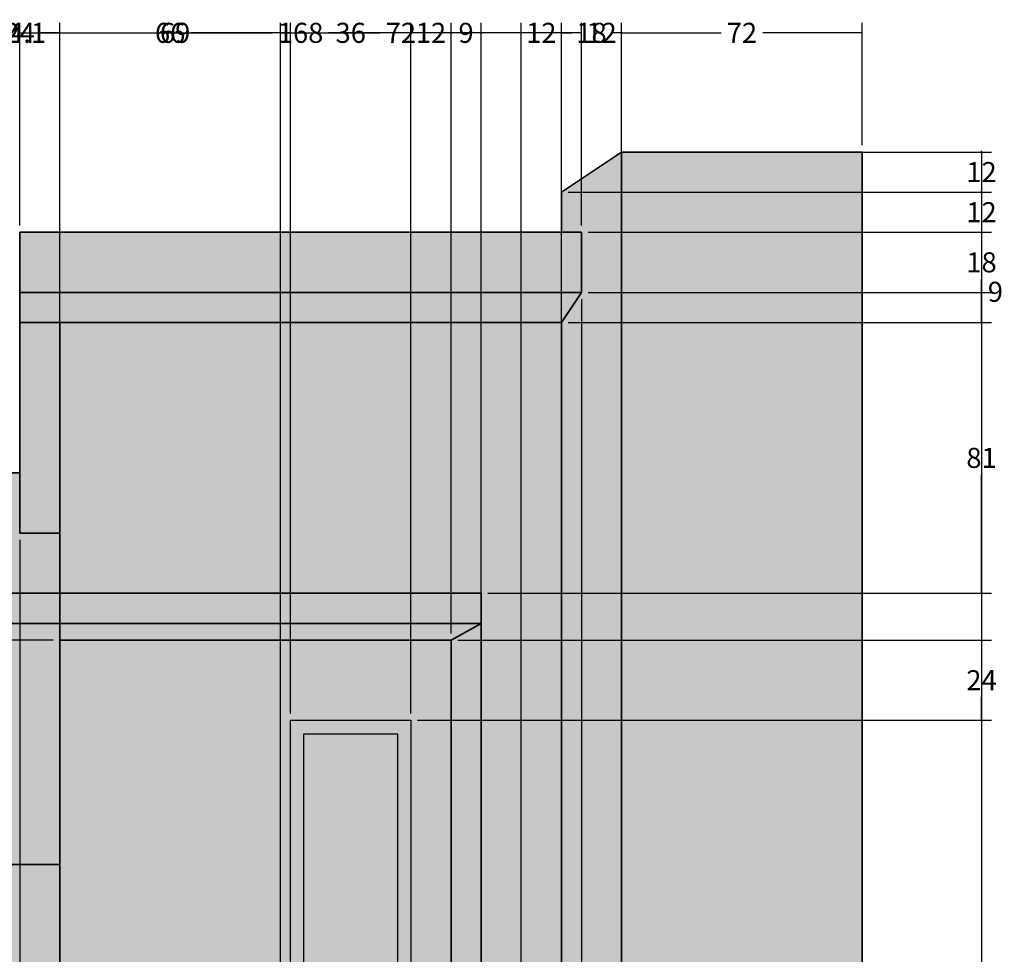
# Model space of a CAD drawing. Units: inches. Extents: x 860 to 1491, y 583 to 1370.
# Tile 8 of 8: x 1190 to 1485, y 1091 to 1370. Entities that reach past the tile are written whole.
import ezdxf

# ---------------------------------------------------------------- set-up
doc = ezdxf.new("R2010")
doc.units = ezdxf.units.IN
doc.header["$MEASUREMENT"] = 0
doc.layers.get('0').update_dxf_attribs({"color": 250})
for name, color, linetype, lineweight in [('A-ANNO-DIMS', 2, 'Continuous', 18), ('A-ELEV', 7, 'Continuous', 35), ('A-ELEV-PATT', 9, 'Continuous', 13), ('A-GLAZ', 4, 'Continuous', 25), ('A-GLAZ-PATT', 150, 'Continuous', 13)]:
    doc.layers.add(name, color=color, linetype=linetype, lineweight=lineweight)
doc.styles.get("Standard").update_dxf_attribs({"font": 'arial.ttf'})
doc.dimstyles.get("Standard").update_dxf_attribs({"dimtxt": 6, "dimasz": 0.18, "dimexe": 3, "dimexo": 2, "dimgap": 2, "dimtad": 0, "dimtih": 1, "dimtoh": 1, "dimdec": 0, "dimzin": 0, "dimdsep": 46, "dimlunit": 3, "dimtxsty": 'Standard', "dimblk2": 'CLOSEDBLANK', "dimsah": 1, "dimcen": 2, "dimadec": 0, "dimazin": 0, "dimtfac": 1, "dimtdec": 0, "dimtofl": 0, "dimtmove": 0, "dimatfit": 3, "dimfxl": 1, "dimtolj": 1, "dimtzin": 0, "dimarcsym": 0})

# ---------------------------------------------------------------- blocks, each defined once
blk = doc.blocks.new('_ClosedBlank')
at = {"color": 0, "linetype": 'ByBlock', "lineweight": -2}
for p, q in [((-1, 0.17), (0, 0)), ((-1, 0.17), (-1, -0.17)), ((0, 0), (-1, -0.17))]:
    blk.add_line(p, q, dxfattribs=at)
blk = doc.blocks.new('*D2')
at = {"layer": 'A-ANNO-DIMS', "color": 0, "lineweight": -2, "transparency": 16777216}
for p, q in [((1442.44, 1328.76), (1442.44, 584.11)), ((908.34, 740.76), (908.34, 584.11)), ((908.52, 587.11), (1163.85, 587.11)), ((1442.26, 587.11), (1186.93, 587.11))]:
    blk.add_line(p, q, dxfattribs=at)
at = {"layer": 'A-ANNO-DIMS', "color": 0, "transparency": 16777216}
blk.add_solid([(908.52, 587.14), (908.52, 587.08), (908.34, 587.11)], dxfattribs=at)
at = {"layer": 'Defpoints', "color": 0, "transparency": 16777216}
for p in [(1442.44, 1330.76), (908.34, 742.76), (1442.44, 587.11)]:
    blk.add_point(p, dxfattribs=at)
at = {"layer": 'A-ANNO-DIMS', "color": 0, "lineweight": -2, "transparency": 16777216, "xscale": 0.18, "yscale": 0.18, "zscale": 0.18}
blk.add_blockref('_ClosedBlank', (1442.44, 587.11), dxfattribs=at)
at = {"layer": 'A-ANNO-DIMS', "color": 0, "transparency": 16777216, "insert": (1175.39, 587.11), "char_height": 6, "attachment_point": 5}
blk.add_mtext('\\A1;534.1', dxfattribs=at)
blk = doc.blocks.new('*D3')
at = {"layer": 'A-ANNO-DIMS', "color": 0, "lineweight": -2, "transparency": 16777216}
for p, q in [((1444.44, 1330.76), (1481.09, 1330.76)), ((1478.09, 1330.58), (1478.09, 981.82)), ((1478.09, 622.94), (1478.09, 971.69)), ((1444.44, 622.76), (1481.09, 622.76))]:
    blk.add_line(p, q, dxfattribs=at)
at = {"layer": 'A-ANNO-DIMS', "color": 0, "transparency": 16777216}
blk.add_solid([(1478.06, 622.94), (1478.12, 622.94), (1478.09, 622.76)], dxfattribs=at)
at = {"layer": 'Defpoints', "color": 0, "transparency": 16777216}
for p in [(1442.44, 1330.76), (1478.09, 1330.76), (1442.44, 622.76)]:
    blk.add_point(p, dxfattribs=at)
at = {"layer": 'A-ANNO-DIMS', "color": 0, "lineweight": -2, "transparency": 16777216, "xscale": 0.18, "yscale": 0.18, "zscale": 0.18, "rotation": 90}
blk.add_blockref('_ClosedBlank', (1478.09, 1330.76), dxfattribs=at)
at = {"layer": 'A-ANNO-DIMS', "color": 0, "transparency": 16777216, "insert": (1478.09, 976.76), "char_height": 6, "attachment_point": 5}
blk.add_mtext('\\A1;708', dxfattribs=at)
blk = doc.blocks.new('*D25')
at = {"layer": 'A-ANNO-DIMS', "color": 0, "lineweight": -2, "transparency": 16777216}
for p, q in [((1178.44, 840.76), (1178.44, 1369.41)), ((1202.44, 744.76), (1202.44, 1369.41)), ((1178.62, 1366.41), (1184.1, 1366.41)), ((1202.26, 1366.41), (1196.78, 1366.41))]:
    blk.add_line(p, q, dxfattribs=at)
at = {"layer": 'A-ANNO-DIMS', "color": 0, "transparency": 16777216}
blk.add_solid([(1178.62, 1366.44), (1178.62, 1366.38), (1178.44, 1366.41)], dxfattribs=at)
at = {"layer": 'Defpoints', "color": 0, "transparency": 16777216}
for p in [(1202.44, 1366.41), (1178.44, 838.76), (1202.44, 742.76)]:
    blk.add_point(p, dxfattribs=at)
at = {"layer": 'A-ANNO-DIMS', "color": 0, "lineweight": -2, "transparency": 16777216, "xscale": 0.18, "yscale": 0.18, "zscale": 0.18}
blk.add_blockref('_ClosedBlank', (1202.44, 1366.41), dxfattribs=at)
at = {"layer": 'A-ANNO-DIMS', "color": 0, "transparency": 16777216, "insert": (1190.44, 1366.41), "char_height": 6, "attachment_point": 5}
blk.add_mtext('\\A1;24', dxfattribs=at)
blk = doc.blocks.new('*D26')
at = {"layer": 'A-ANNO-DIMS', "color": 0, "lineweight": -2, "transparency": 16777216}
for p, q in [((1202.44, 744.76), (1202.44, 1369.41)), ((1268.44, 864.76), (1268.44, 1369.41)), ((1202.62, 1366.41), (1229.13, 1366.41)), ((1268.26, 1366.41), (1241.75, 1366.41))]:
    blk.add_line(p, q, dxfattribs=at)
at = {"layer": 'A-ANNO-DIMS', "color": 0, "transparency": 16777216}
blk.add_solid([(1202.62, 1366.44), (1202.62, 1366.38), (1202.44, 1366.41)], dxfattribs=at)
at = {"layer": 'Defpoints', "color": 0, "transparency": 16777216}
for p in [(1268.44, 1366.41), (1268.44, 862.76), (1202.44, 742.76)]:
    blk.add_point(p, dxfattribs=at)
at = {"layer": 'A-ANNO-DIMS', "color": 0, "lineweight": -2, "transparency": 16777216, "xscale": 0.18, "yscale": 0.18, "zscale": 0.18}
blk.add_blockref('_ClosedBlank', (1268.44, 1366.41), dxfattribs=at)
at = {"layer": 'A-ANNO-DIMS', "color": 0, "transparency": 16777216, "insert": (1235.44, 1366.41), "char_height": 6, "attachment_point": 5}
blk.add_mtext('\\A1;66', dxfattribs=at)
blk = doc.blocks.new('*D27')
at = {"layer": 'A-ANNO-DIMS', "color": 0, "lineweight": -2, "transparency": 16777216}
for p, q in [((1268.44, 864.76), (1268.44, 1369.41)), ((1340.44, 864.76), (1340.44, 1369.41)), ((1268.62, 1366.41), (1298.2, 1366.41)), ((1340.26, 1366.41), (1310.68, 1366.41))]:
    blk.add_line(p, q, dxfattribs=at)
at = {"layer": 'A-ANNO-DIMS', "color": 0, "transparency": 16777216}
blk.add_solid([(1268.62, 1366.44), (1268.62, 1366.38), (1268.44, 1366.41)], dxfattribs=at)
at = {"layer": 'Defpoints', "color": 0, "transparency": 16777216}
for p in [(1340.44, 1366.41), (1268.44, 862.76), (1340.44, 862.76)]:
    blk.add_point(p, dxfattribs=at)
at = {"layer": 'A-ANNO-DIMS', "color": 0, "lineweight": -2, "transparency": 16777216, "xscale": 0.18, "yscale": 0.18, "zscale": 0.18}
blk.add_blockref('_ClosedBlank', (1340.44, 1366.41), dxfattribs=at)
at = {"layer": 'A-ANNO-DIMS', "color": 0, "transparency": 16777216, "insert": (1304.44, 1366.41), "char_height": 6, "attachment_point": 5}
blk.add_mtext('\\A1;72', dxfattribs=at)
blk = doc.blocks.new('*D28')
at = {"layer": 'A-ANNO-DIMS', "color": 0, "lineweight": -2, "transparency": 16777216}
for p, q in [((1340.440309, 864.755507), (1340.440309, 1369.405507)), ((1352.440309, 732.755507), (1352.440309, 1369.405507)), ((1340.260309, 1366.405507), (1340.080309, 1366.405507)), ((1352.620309, 1366.405507), (1352.800309, 1366.405507))]:
    blk.add_line(p, q, dxfattribs=at)
at = {"layer": 'A-ANNO-DIMS', "color": 0, "transparency": 16777216}
blk.add_solid([(1340.260309, 1366.435507), (1340.260309, 1366.375507), (1340.440309, 1366.405507)], dxfattribs=at)
at = {"layer": 'Defpoints', "color": 0, "transparency": 16777216}
for p in [(1352.440309, 1366.405507), (1340.440309, 862.755507), (1352.440309, 730.755507)]:
    blk.add_point(p, dxfattribs=at)
at = {"layer": 'A-ANNO-DIMS', "color": 0, "lineweight": -2, "transparency": 16777216, "xscale": 0.18, "yscale": 0.18, "zscale": 0.18, "rotation": 180}
blk.add_blockref('_ClosedBlank', (1352.440309, 1366.405507), dxfattribs=at)
at = {"layer": 'A-ANNO-DIMS', "color": 0, "transparency": 16777216, "insert": (1346.440309, 1366.405507), "char_height": 6, "attachment_point": 5}
blk.add_mtext('\\A1;12', dxfattribs=at)
blk = doc.blocks.new('*D29')
at = {"layer": 'A-ANNO-DIMS', "color": 0, "lineweight": -2, "transparency": 16777216}
for p, q in [((1352.44, 732.76), (1352.44, 1369.41)), ((1370.44, 732.76), (1370.44, 1369.41)), ((1352.62, 1366.41), (1355.42, 1366.41)), ((1370.26, 1366.41), (1367.46, 1366.41))]:
    blk.add_line(p, q, dxfattribs=at)
at = {"layer": 'A-ANNO-DIMS', "color": 0, "transparency": 16777216}
blk.add_solid([(1352.62, 1366.44), (1352.62, 1366.38), (1352.44, 1366.41)], dxfattribs=at)
at = {"layer": 'Defpoints', "color": 0, "transparency": 16777216}
for p in [(1370.44, 1366.41), (1352.44, 730.76), (1370.44, 730.76)]:
    blk.add_point(p, dxfattribs=at)
at = {"layer": 'A-ANNO-DIMS', "color": 0, "lineweight": -2, "transparency": 16777216, "xscale": 0.18, "yscale": 0.18, "zscale": 0.18}
blk.add_blockref('_ClosedBlank', (1370.44, 1366.41), dxfattribs=at)
at = {"layer": 'A-ANNO-DIMS', "color": 0, "transparency": 16777216, "insert": (1361.44, 1366.41), "char_height": 6, "attachment_point": 5}
blk.add_mtext('\\A1;18', dxfattribs=at)
blk = doc.blocks.new('*D47')
at = {"layer": 'A-ANNO-DIMS', "color": 0, "lineweight": -2, "transparency": 16777216}
for p, q in [((1200.44, 1184.76), (869.69, 1184.76)), ((872.69, 1184.58), (872.69, 1156.25)), ((872.69, 1117.8), (872.69, 1146.12)), ((960.34, 1117.62), (869.69, 1117.62))]:
    blk.add_line(p, q, dxfattribs=at)
at = {"layer": 'A-ANNO-DIMS', "color": 0, "transparency": 16777216}
blk.add_solid([(872.66, 1117.8), (872.72, 1117.8), (872.69, 1117.62)], dxfattribs=at)
at = {"layer": 'Defpoints', "color": 0, "transparency": 16777216}
for p in [(872.69, 1184.76), (1202.44, 1184.76), (962.34, 1117.62)]:
    blk.add_point(p, dxfattribs=at)
at = {"layer": 'A-ANNO-DIMS', "color": 0, "lineweight": -2, "transparency": 16777216, "xscale": 0.18, "yscale": 0.18, "zscale": 0.18, "rotation": 90}
blk.add_blockref('_ClosedBlank', (872.69, 1184.76), dxfattribs=at)
at = {"layer": 'A-ANNO-DIMS', "color": 0, "transparency": 16777216, "insert": (872.69, 1151.19), "char_height": 6, "attachment_point": 5}
blk.add_mtext('\\A1;67.13', dxfattribs=at)
blk = doc.blocks.new('*D53')
at = {"layer": 'A-ANNO-DIMS', "color": 0, "lineweight": -2, "transparency": 16777216}
for p, q in [((1309.44, 1160.76), (1481.09, 1160.76)), ((1478.09, 1160.58), (1478.09, 1057.82)), ((1478.09, 944.94), (1478.09, 1047.69)), ((1309.44, 944.76), (1481.09, 944.76))]:
    blk.add_line(p, q, dxfattribs=at)
at = {"layer": 'A-ANNO-DIMS', "color": 0, "transparency": 16777216}
blk.add_solid([(1478.06, 944.94), (1478.12, 944.94), (1478.09, 944.76)], dxfattribs=at)
at = {"layer": 'Defpoints', "color": 0, "transparency": 16777216}
for p in [(1307.44, 1160.76), (1478.09, 1160.76), (1307.44, 944.76)]:
    blk.add_point(p, dxfattribs=at)
at = {"layer": 'A-ANNO-DIMS', "color": 0, "lineweight": -2, "transparency": 16777216, "xscale": 0.18, "yscale": 0.18, "zscale": 0.18, "rotation": 90}
blk.add_blockref('_ClosedBlank', (1478.09, 1160.76), dxfattribs=at)
at = {"layer": 'A-ANNO-DIMS', "color": 0, "transparency": 16777216, "insert": (1478.09, 1052.76), "char_height": 6, "attachment_point": 5}
blk.add_mtext('\\A1;216', dxfattribs=at)
blk = doc.blocks.new('*D54')
at = {"layer": 'A-ANNO-DIMS', "color": 0, "lineweight": -2, "transparency": 16777216}
for p, q in [((1321.44, 1184.76), (1481.09, 1184.76)), ((1478.09, 1184.58), (1478.09, 1177.77)), ((1478.09, 1160.94), (1478.09, 1167.74)), ((1309.44, 1160.76), (1481.09, 1160.76))]:
    blk.add_line(p, q, dxfattribs=at)
at = {"layer": 'A-ANNO-DIMS', "color": 0, "transparency": 16777216}
blk.add_solid([(1478.06, 1160.94), (1478.12, 1160.94), (1478.09, 1160.76)], dxfattribs=at)
at = {"layer": 'Defpoints', "color": 0, "transparency": 16777216}
for p in [(1319.44, 1184.76), (1478.09, 1184.76), (1307.44, 1160.76)]:
    blk.add_point(p, dxfattribs=at)
at = {"layer": 'A-ANNO-DIMS', "color": 0, "lineweight": -2, "transparency": 16777216, "xscale": 0.18, "yscale": 0.18, "zscale": 0.18, "rotation": 90}
blk.add_blockref('_ClosedBlank', (1478.09, 1184.76), dxfattribs=at)
at = {"layer": 'A-ANNO-DIMS', "color": 0, "transparency": 16777216, "insert": (1478.09, 1172.76), "char_height": 6, "attachment_point": 5}
blk.add_mtext('\\A1;24', dxfattribs=at)
blk = doc.blocks.new('*D57')
at = {"layer": 'A-ANNO-DIMS', "color": 0, "lineweight": -2, "transparency": 16777216}
for p, q in [((1178.34, 1092.76), (1178.34, 1369.41)), ((1202.44, 1186.76), (1202.44, 1369.41)), ((1178.52, 1366.41), (1181.13, 1366.41)), ((1202.26, 1366.41), (1199.65, 1366.41))]:
    blk.add_line(p, q, dxfattribs=at)
at = {"layer": 'A-ANNO-DIMS', "color": 0, "transparency": 16777216}
blk.add_solid([(1178.52, 1366.44), (1178.52, 1366.38), (1178.34, 1366.41)], dxfattribs=at)
at = {"layer": 'Defpoints', "color": 0, "transparency": 16777216}
for p in [(1202.44, 1366.41), (1202.44, 1184.76), (1178.34, 1090.76)]:
    blk.add_point(p, dxfattribs=at)
at = {"layer": 'A-ANNO-DIMS', "color": 0, "lineweight": -2, "transparency": 16777216, "xscale": 0.18, "yscale": 0.18, "zscale": 0.18}
blk.add_blockref('_ClosedBlank', (1202.44, 1366.41), dxfattribs=at)
at = {"layer": 'A-ANNO-DIMS', "color": 0, "transparency": 16777216, "insert": (1190.39, 1366.41), "char_height": 6, "attachment_point": 5}
blk.add_mtext('\\A1;24.1', dxfattribs=at)
blk = doc.blocks.new('*D58')
at = {"layer": 'A-ANNO-DIMS', "color": 0, "lineweight": -2, "transparency": 16777216}
for p, q in [((1202.44, 1186.76), (1202.44, 1369.41)), ((1271.44, 1162.76), (1271.44, 1369.41)), ((1202.62, 1366.41), (1230.62, 1366.41)), ((1271.26, 1366.41), (1243.26, 1366.41))]:
    blk.add_line(p, q, dxfattribs=at)
at = {"layer": 'A-ANNO-DIMS', "color": 0, "transparency": 16777216}
blk.add_solid([(1202.62, 1366.44), (1202.62, 1366.38), (1202.44, 1366.41)], dxfattribs=at)
at = {"layer": 'Defpoints', "color": 0, "transparency": 16777216}
for p in [(1271.44, 1366.41), (1202.44, 1184.76), (1271.44, 1160.76)]:
    blk.add_point(p, dxfattribs=at)
at = {"layer": 'A-ANNO-DIMS', "color": 0, "lineweight": -2, "transparency": 16777216, "xscale": 0.18, "yscale": 0.18, "zscale": 0.18}
blk.add_blockref('_ClosedBlank', (1271.44, 1366.41), dxfattribs=at)
at = {"layer": 'A-ANNO-DIMS', "color": 0, "transparency": 16777216, "insert": (1236.94, 1366.41), "char_height": 6, "attachment_point": 5}
blk.add_mtext('\\A1;69', dxfattribs=at)
blk = doc.blocks.new('*D59')
at = {"layer": 'A-ANNO-DIMS', "color": 0, "lineweight": -2, "transparency": 16777216}
for p, q in [((1271.44, 1162.76), (1271.44, 1369.41)), ((1307.44, 1162.76), (1307.44, 1369.41)), ((1271.62, 1366.41), (1283.15, 1366.41)), ((1307.26, 1366.41), (1295.73, 1366.41))]:
    blk.add_line(p, q, dxfattribs=at)
at = {"layer": 'A-ANNO-DIMS', "color": 0, "transparency": 16777216}
blk.add_solid([(1271.62, 1366.44), (1271.62, 1366.38), (1271.44, 1366.41)], dxfattribs=at)
at = {"layer": 'Defpoints', "color": 0, "transparency": 16777216}
for p in [(1307.44, 1366.41), (1271.44, 1160.76), (1307.44, 1160.76)]:
    blk.add_point(p, dxfattribs=at)
at = {"layer": 'A-ANNO-DIMS', "color": 0, "lineweight": -2, "transparency": 16777216, "xscale": 0.18, "yscale": 0.18, "zscale": 0.18}
blk.add_blockref('_ClosedBlank', (1307.44, 1366.41), dxfattribs=at)
at = {"layer": 'A-ANNO-DIMS', "color": 0, "transparency": 16777216, "insert": (1289.44, 1366.41), "char_height": 6, "attachment_point": 5}
blk.add_mtext('\\A1;36', dxfattribs=at)
blk = doc.blocks.new('*D60')
at = {"layer": 'A-ANNO-DIMS', "color": 0, "lineweight": -2, "transparency": 16777216}
for p, q in [((1307.440309, 1162.755507), (1307.440309, 1369.405507)), ((1319.440309, 1186.755507), (1319.440309, 1369.405507)), ((1307.260309, 1366.405507), (1307.080309, 1366.405507)), ((1319.620309, 1366.405507), (1319.800309, 1366.405507))]:
    blk.add_line(p, q, dxfattribs=at)
at = {"layer": 'A-ANNO-DIMS', "color": 0, "transparency": 16777216}
blk.add_solid([(1307.260309, 1366.435507), (1307.260309, 1366.375507), (1307.440309, 1366.405507)], dxfattribs=at)
at = {"layer": 'Defpoints', "color": 0, "transparency": 16777216}
for p in [(1319.440309, 1366.405507), (1319.440309, 1184.755507), (1307.440309, 1160.755507)]:
    blk.add_point(p, dxfattribs=at)
at = {"layer": 'A-ANNO-DIMS', "color": 0, "lineweight": -2, "transparency": 16777216, "xscale": 0.18, "yscale": 0.18, "zscale": 0.18, "rotation": 180}
blk.add_blockref('_ClosedBlank', (1319.440309, 1366.405507), dxfattribs=at)
at = {"layer": 'A-ANNO-DIMS', "color": 0, "transparency": 16777216, "insert": (1313.440309, 1366.405507), "char_height": 6, "attachment_point": 5}
blk.add_mtext('\\A1;12', dxfattribs=at)
blk = doc.blocks.new('*D61')
at = {"layer": 'A-ANNO-DIMS', "color": 0, "lineweight": -2, "transparency": 16777216}
for p, q in [((1319.440309, 1186.755507), (1319.440309, 1369.405507)), ((1328.440309, 924.755507), (1328.440309, 1369.405507)), ((1319.260309, 1366.405507), (1319.080309, 1366.405507)), ((1328.620309, 1366.405507), (1328.800309, 1366.405507))]:
    blk.add_line(p, q, dxfattribs=at)
at = {"layer": 'A-ANNO-DIMS', "color": 0, "transparency": 16777216}
blk.add_solid([(1319.260309, 1366.435507), (1319.260309, 1366.375507), (1319.440309, 1366.405507)], dxfattribs=at)
at = {"layer": 'Defpoints', "color": 0, "transparency": 16777216}
for p in [(1328.440309, 1366.405507), (1319.440309, 1184.755507), (1328.440309, 922.755507)]:
    blk.add_point(p, dxfattribs=at)
at = {"layer": 'A-ANNO-DIMS', "color": 0, "lineweight": -2, "transparency": 16777216, "xscale": 0.18, "yscale": 0.18, "zscale": 0.18, "rotation": 180}
blk.add_blockref('_ClosedBlank', (1328.440309, 1366.405507), dxfattribs=at)
at = {"layer": 'A-ANNO-DIMS', "color": 0, "transparency": 16777216, "insert": (1323.940309, 1366.405507), "char_height": 6, "attachment_point": 5}
blk.add_mtext('\\A1;9', dxfattribs=at)
blk = doc.blocks.new('*D73')
at = {"layer": 'A-ANNO-DIMS', "color": 0, "lineweight": -2, "transparency": 16777216}
for p, q in [((1190.44, 1308.76), (1190.44, 1369.41)), ((1358.44, 1308.76), (1358.44, 1369.41)), ((1190.62, 1366.41), (1266.09, 1366.41)), ((1358.26, 1366.41), (1282.79, 1366.41))]:
    blk.add_line(p, q, dxfattribs=at)
at = {"layer": 'A-ANNO-DIMS', "color": 0, "transparency": 16777216}
blk.add_solid([(1190.62, 1366.44), (1190.62, 1366.38), (1190.44, 1366.41)], dxfattribs=at)
at = {"layer": 'Defpoints', "color": 0, "transparency": 16777216}
for p in [(1358.44, 1366.41), (1190.44, 1306.76), (1358.44, 1306.76)]:
    blk.add_point(p, dxfattribs=at)
at = {"layer": 'A-ANNO-DIMS', "color": 0, "lineweight": -2, "transparency": 16777216, "xscale": 0.18, "yscale": 0.18, "zscale": 0.18}
blk.add_blockref('_ClosedBlank', (1358.44, 1366.41), dxfattribs=at)
at = {"layer": 'A-ANNO-DIMS', "color": 0, "transparency": 16777216, "insert": (1274.44, 1366.41), "char_height": 6, "attachment_point": 5}
blk.add_mtext('\\A1;168', dxfattribs=at)
blk = doc.blocks.new('*D74')
at = {"layer": 'A-ANNO-DIMS', "color": 0, "lineweight": -2, "transparency": 16777216}
for p, q in [((1358.440309, 1308.755507), (1358.440309, 1369.405507)), ((1370.440309, 1332.755507), (1370.440309, 1369.405507)), ((1358.260309, 1366.405507), (1358.080309, 1366.405507)), ((1370.620309, 1366.405507), (1370.800309, 1366.405507))]:
    blk.add_line(p, q, dxfattribs=at)
at = {"layer": 'A-ANNO-DIMS', "color": 0, "transparency": 16777216}
blk.add_solid([(1358.260309, 1366.435507), (1358.260309, 1366.375507), (1358.440309, 1366.405507)], dxfattribs=at)
at = {"layer": 'Defpoints', "color": 0, "transparency": 16777216}
for p in [(1370.440309, 1366.405507), (1370.440309, 1330.755507), (1358.440309, 1306.755507)]:
    blk.add_point(p, dxfattribs=at)
at = {"layer": 'A-ANNO-DIMS', "color": 0, "lineweight": -2, "transparency": 16777216, "xscale": 0.18, "yscale": 0.18, "zscale": 0.18, "rotation": 180}
blk.add_blockref('_ClosedBlank', (1370.440309, 1366.405507), dxfattribs=at)
at = {"layer": 'A-ANNO-DIMS', "color": 0, "transparency": 16777216, "insert": (1364.440309, 1366.405507), "char_height": 6, "attachment_point": 5}
blk.add_mtext('\\A1;12', dxfattribs=at)
blk = doc.blocks.new('*D75')
at = {"layer": 'A-ANNO-DIMS', "color": 0, "lineweight": -2, "transparency": 16777216}
for p, q in [((1370.44, 1332.76), (1370.44, 1369.41)), ((1442.44, 1332.76), (1442.44, 1369.41)), ((1370.62, 1366.41), (1400.2, 1366.41)), ((1442.26, 1366.41), (1412.68, 1366.41))]:
    blk.add_line(p, q, dxfattribs=at)
at = {"layer": 'A-ANNO-DIMS', "color": 0, "transparency": 16777216}
blk.add_solid([(1370.62, 1366.44), (1370.62, 1366.38), (1370.44, 1366.41)], dxfattribs=at)
at = {"layer": 'Defpoints', "color": 0, "transparency": 16777216}
for p in [(1442.44, 1366.41), (1370.44, 1330.76), (1442.44, 1330.76)]:
    blk.add_point(p, dxfattribs=at)
at = {"layer": 'A-ANNO-DIMS', "color": 0, "lineweight": -2, "transparency": 16777216, "xscale": 0.18, "yscale": 0.18, "zscale": 0.18}
blk.add_blockref('_ClosedBlank', (1442.44, 1366.41), dxfattribs=at)
at = {"layer": 'A-ANNO-DIMS', "color": 0, "transparency": 16777216, "insert": (1406.44, 1366.41), "char_height": 6, "attachment_point": 5}
blk.add_mtext('\\A1;72', dxfattribs=at)
blk = doc.blocks.new('*D76')
at = {"layer": 'A-ANNO-DIMS', "color": 0, "lineweight": -2, "transparency": 16777216}
for p, q in [((1202.440309, 1277.755507), (1202.440309, 584.105507)), ((1190.440309, 1214.755507), (1190.440309, 584.105507)), ((1190.260309, 587.105507), (1190.080309, 587.105507)), ((1202.620309, 587.105507), (1202.800309, 587.105507))]:
    blk.add_line(p, q, dxfattribs=at)
at = {"layer": 'A-ANNO-DIMS', "color": 0, "transparency": 16777216}
blk.add_solid([(1190.260309, 587.135507), (1190.260309, 587.075507), (1190.440309, 587.105507)], dxfattribs=at)
at = {"layer": 'Defpoints', "color": 0, "transparency": 16777216}
for p in [(1202.440309, 1279.755507), (1190.440309, 1216.755507), (1202.440309, 587.105507)]:
    blk.add_point(p, dxfattribs=at)
at = {"layer": 'A-ANNO-DIMS', "color": 0, "lineweight": -2, "transparency": 16777216, "xscale": 0.18, "yscale": 0.18, "zscale": 0.18, "rotation": 180}
blk.add_blockref('_ClosedBlank', (1202.440309, 587.105507), dxfattribs=at)
at = {"layer": 'A-ANNO-DIMS', "color": 0, "transparency": 16777216, "insert": (1196.440309, 587.105507), "char_height": 6, "attachment_point": 5}
blk.add_mtext('\\A1;12', dxfattribs=at)
blk = doc.blocks.new('*D77')
at = {"layer": 'A-ANNO-DIMS', "color": 0, "lineweight": -2, "transparency": 16777216}
for p, q in [((1202.44, 1277.76), (1202.44, 584.11)), ((1352.44, 1277.76), (1352.44, 584.11)), ((1202.62, 587.11), (1269.1, 587.11)), ((1352.26, 587.11), (1285.78, 587.11))]:
    blk.add_line(p, q, dxfattribs=at)
at = {"layer": 'A-ANNO-DIMS', "color": 0, "transparency": 16777216}
blk.add_solid([(1202.62, 587.14), (1202.62, 587.08), (1202.44, 587.11)], dxfattribs=at)
at = {"layer": 'Defpoints', "color": 0, "transparency": 16777216}
for p in [(1202.44, 1279.76), (1352.44, 1279.76), (1352.44, 587.11)]:
    blk.add_point(p, dxfattribs=at)
at = {"layer": 'A-ANNO-DIMS', "color": 0, "lineweight": -2, "transparency": 16777216, "xscale": 0.18, "yscale": 0.18, "zscale": 0.18}
blk.add_blockref('_ClosedBlank', (1352.44, 587.11), dxfattribs=at)
at = {"layer": 'A-ANNO-DIMS', "color": 0, "transparency": 16777216, "insert": (1277.44, 587.11), "char_height": 6, "attachment_point": 5}
blk.add_mtext('\\A1;150', dxfattribs=at)
blk = doc.blocks.new('*D78')
at = {"layer": 'A-ANNO-DIMS', "color": 0, "lineweight": -2, "transparency": 16777216}
for p, q in [((1358.44, 1286.76), (1358.44, 584.11)), ((1352.44, 1277.76), (1352.44, 584.11)), ((1352.62, 587.11), (1358.26, 587.11)), ((1358.44, 587.11), (1358.62, 587.11))]:
    blk.add_line(p, q, dxfattribs=at)
at = {"layer": 'A-ANNO-DIMS', "color": 0, "transparency": 16777216}
blk.add_solid([(1352.62, 587.14), (1352.62, 587.08), (1352.44, 587.11)], dxfattribs=at)
at = {"layer": 'Defpoints', "color": 0, "transparency": 16777216}
for p in [(1358.44, 1288.76), (1352.44, 1279.76), (1358.44, 587.11)]:
    blk.add_point(p, dxfattribs=at)
at = {"layer": 'A-ANNO-DIMS', "color": 0, "lineweight": -2, "transparency": 16777216, "xscale": 0.18, "yscale": 0.18, "zscale": 0.18}
blk.add_blockref('_ClosedBlank', (1358.44, 587.11), dxfattribs=at)
at = {"layer": 'A-ANNO-DIMS', "color": 0, "transparency": 16777216, "insert": (1362.6, 587.11), "char_height": 6, "attachment_point": 5}
blk.add_mtext('\\A1;6', dxfattribs=at)
blk = doc.blocks.new('*D82')
at = {"layer": 'A-ANNO-DIMS', "color": 0, "lineweight": -2, "transparency": 16777216}
for p, q in [((1354.44, 1279.76), (1481.09, 1279.76)), ((1478.09, 1279.58), (1478.09, 1244.32)), ((1478.09, 1198.94), (1478.09, 1234.19)), ((1330.44, 1198.76), (1481.09, 1198.76))]:
    blk.add_line(p, q, dxfattribs=at)
at = {"layer": 'A-ANNO-DIMS', "color": 0, "transparency": 16777216}
blk.add_solid([(1478.06, 1198.94), (1478.12, 1198.94), (1478.09, 1198.76)], dxfattribs=at)
at = {"layer": 'Defpoints', "color": 0, "transparency": 16777216}
for p in [(1352.44, 1279.76), (1478.09, 1279.76), (1328.44, 1198.76)]:
    blk.add_point(p, dxfattribs=at)
at = {"layer": 'A-ANNO-DIMS', "color": 0, "lineweight": -2, "transparency": 16777216, "xscale": 0.18, "yscale": 0.18, "zscale": 0.18, "rotation": 90}
blk.add_blockref('_ClosedBlank', (1478.09, 1279.76), dxfattribs=at)
at = {"layer": 'A-ANNO-DIMS', "color": 0, "transparency": 16777216, "insert": (1478.09, 1239.26), "char_height": 6, "attachment_point": 5}
blk.add_mtext('\\A1;81', dxfattribs=at)
blk = doc.blocks.new('*D83')
at = {"layer": 'A-ANNO-DIMS', "color": 0, "lineweight": -2, "transparency": 16777216}
for p, q in [((1360.44, 1288.76), (1481.09, 1288.76)), ((1478.09, 1288.76), (1478.09, 1288.94)), ((1478.09, 1288.94), (1478.27, 1288.94)), ((1478.09, 1279.94), (1478.09, 1288.58)), ((1354.44, 1279.76), (1481.09, 1279.76))]:
    blk.add_line(p, q, dxfattribs=at)
at = {"layer": 'A-ANNO-DIMS', "color": 0, "transparency": 16777216}
blk.add_solid([(1478.06, 1279.94), (1478.12, 1279.94), (1478.09, 1279.76)], dxfattribs=at)
at = {"layer": 'Defpoints', "color": 0, "transparency": 16777216}
for p in [(1358.44, 1288.76), (1478.09, 1288.76), (1352.44, 1279.76)]:
    blk.add_point(p, dxfattribs=at)
at = {"layer": 'A-ANNO-DIMS', "color": 0, "lineweight": -2, "transparency": 16777216, "xscale": 0.18, "yscale": 0.18, "zscale": 0.18, "rotation": 90}
blk.add_blockref('_ClosedBlank', (1478.09, 1288.76), dxfattribs=at)
at = {"layer": 'A-ANNO-DIMS', "color": 0, "transparency": 16777216, "insert": (1482.24, 1288.94), "char_height": 6, "attachment_point": 5}
blk.add_mtext('\\A1;9', dxfattribs=at)
blk = doc.blocks.new('*D84')
at = {"layer": 'A-ANNO-DIMS', "color": 0, "lineweight": -2, "transparency": 16777216}
for p, q in [((1360.44, 1306.76), (1481.09, 1306.76)), ((1478.09, 1306.58), (1478.09, 1302.82)), ((1478.09, 1288.94), (1478.09, 1292.69)), ((1360.44, 1288.76), (1481.09, 1288.76))]:
    blk.add_line(p, q, dxfattribs=at)
at = {"layer": 'A-ANNO-DIMS', "color": 0, "transparency": 16777216}
blk.add_solid([(1478.06, 1288.94), (1478.12, 1288.94), (1478.09, 1288.76)], dxfattribs=at)
at = {"layer": 'Defpoints', "color": 0, "transparency": 16777216}
for p in [(1358.44, 1306.76), (1478.09, 1306.76), (1358.44, 1288.76)]:
    blk.add_point(p, dxfattribs=at)
at = {"layer": 'A-ANNO-DIMS', "color": 0, "lineweight": -2, "transparency": 16777216, "xscale": 0.18, "yscale": 0.18, "zscale": 0.18, "rotation": 90}
blk.add_blockref('_ClosedBlank', (1478.09, 1306.76), dxfattribs=at)
at = {"layer": 'A-ANNO-DIMS', "color": 0, "transparency": 16777216, "insert": (1478.09, 1297.76), "char_height": 6, "attachment_point": 5}
blk.add_mtext('\\A1;18', dxfattribs=at)
blk = doc.blocks.new('*D85')
at = {"layer": 'A-ANNO-DIMS', "color": 0, "lineweight": -2, "transparency": 16777216}
for p, q in [((1354.440309, 1318.755507), (1481.090309, 1318.755507)), ((1478.090309, 1318.935507), (1478.090309, 1319.115507)), ((1360.440309, 1306.755507), (1481.090309, 1306.755507)), ((1478.090309, 1306.575507), (1478.090309, 1306.395507))]:
    blk.add_line(p, q, dxfattribs=at)
at = {"layer": 'A-ANNO-DIMS', "color": 0, "transparency": 16777216}
blk.add_solid([(1478.060309, 1306.575507), (1478.120309, 1306.575507), (1478.090309, 1306.755507)], dxfattribs=at)
at = {"layer": 'Defpoints', "color": 0, "transparency": 16777216}
for p in [(1352.440309, 1318.755507), (1478.090309, 1318.755507), (1358.440309, 1306.755507)]:
    blk.add_point(p, dxfattribs=at)
at = {"layer": 'A-ANNO-DIMS', "color": 0, "lineweight": -2, "transparency": 16777216, "xscale": 0.18, "yscale": 0.18, "zscale": 0.18, "rotation": 270}
blk.add_blockref('_ClosedBlank', (1478.090309, 1318.755507), dxfattribs=at)
at = {"layer": 'A-ANNO-DIMS', "color": 0, "transparency": 16777216, "insert": (1478.090309, 1312.755507), "char_height": 6, "attachment_point": 5}
blk.add_mtext('\\A1;12', dxfattribs=at)
blk = doc.blocks.new('*D86')
at = {"layer": 'A-ANNO-DIMS', "color": 0, "lineweight": -2, "transparency": 16777216}
for p, q in [((1478.090309, 1330.935507), (1478.090309, 1331.115507)), ((1372.440309, 1330.755507), (1481.090309, 1330.755507)), ((1354.440309, 1318.755507), (1481.090309, 1318.755507)), ((1478.090309, 1318.575507), (1478.090309, 1318.395507))]:
    blk.add_line(p, q, dxfattribs=at)
at = {"layer": 'A-ANNO-DIMS', "color": 0, "transparency": 16777216}
blk.add_solid([(1478.060309, 1318.575507), (1478.120309, 1318.575507), (1478.090309, 1318.755507)], dxfattribs=at)
at = {"layer": 'Defpoints', "color": 0, "transparency": 16777216}
for p in [(1370.440309, 1330.755507), (1478.090309, 1330.755507), (1352.440309, 1318.755507)]:
    blk.add_point(p, dxfattribs=at)
at = {"layer": 'A-ANNO-DIMS', "color": 0, "lineweight": -2, "transparency": 16777216, "xscale": 0.18, "yscale": 0.18, "zscale": 0.18, "rotation": 270}
blk.add_blockref('_ClosedBlank', (1478.090309, 1330.755507), dxfattribs=at)
at = {"layer": 'A-ANNO-DIMS', "color": 0, "transparency": 16777216, "insert": (1478.090309, 1324.755507), "char_height": 6, "attachment_point": 5}
blk.add_mtext('\\A1;12', dxfattribs=at)

msp = doc.modelspace()

# ---------------------------------------------------------------- hatches: boundary and pattern name
at = {"layer": 'A-ELEV-PATT'}
h = msp.add_hatch(color=256, dxfattribs=at)
h.dxf.hatch_style = 1
h.paths.add_polyline_path([(1442.4403, 1330.7555), (1370.4403, 1330.7555), (1370.4403, 622.7555), (1442.4403, 622.7555)])
h.paths.add_polyline_path([(1358.4403, 1306.7555), (1190.4403, 1306.7555), (1190.4403, 1288.7555), (1358.4403, 1288.7555)])
h.paths.add_polyline_path([(1190.4403, 1234.7555), (962.3403, 1234.7555), (962.3403, 1198.7555), (1202.4403, 1198.7555), (1202.4403, 1216.7555), (1190.4403, 1216.7555)])
h.paths.add_polyline_path([(1202.4403, 1117.6207), (962.3403, 1117.6207), (962.3403, 982.7555), (986.3403, 982.7555), (986.3403, 1090.7555), (1178.3403, 1090.7555), (1178.3403, 982.7555), (1202.4403, 982.7555)])
h.paths.add_polyline_path([(1319.4403, 1184.7555), (1202.4403, 1184.7555), (1202.4403, 982.7555), (1211.4403, 982.7555), (1211.4403, 946.7555), (1220.4403, 946.7555), (1220.4403, 934.7555), (1319.4403, 934.7555)])
h.paths.add_polyline_path([(1271.4403, 1160.7555), (1307.4403, 1160.7555), (1307.4403, 944.7555), (1271.4403, 944.7555)], flags=16)
h.paths.add_polyline_path([(1275.4403, 1156.7555), (1303.4403, 1156.7555), (1303.4403, 948.7555), (1275.4403, 948.7555)], flags=0)
h.paths.add_polyline_path([(1202.4403, 898.7555), (962.3403, 898.7555), (962.3403, 730.7555), (1034.4585, 730.7555), (1034.4585, 826.7555), (1070.4585, 826.7555), (1070.4585, 730.7555), (1118.4403, 730.7555), (1118.4403, 838.7555), (1178.4403, 838.7555), (1178.4403, 730.7555), (1202.4403, 730.7555)])
h.paths.add_polyline_path([(1220.4403, 946.7555), (1211.4403, 946.7555), (938.3403, 946.7555), (926.3403, 946.7555), (926.3403, 910.7555), (962.3403, 910.7555), (1220.4403, 910.7555)])
h.paths.add_polyline_path([(950.3403, 730.7555), (950.3403, 734.7555), (938.3403, 742.7555), (938.3403, 730.7555), (938.3403, 622.7555), (950.3403, 622.7555)])
h = msp.add_hatch(color=256, dxfattribs=at)
h.dxf.hatch_style = 1
h.paths.add_polyline_path([(1202.4403, 1184.7555), (1319.4403, 1184.7555), (1328.4403, 1189.7555), (938.3403, 1189.7555), (962.3403, 1098.3061), (962.3403, 1117.6207), (1202.4403, 1117.6207)])
h.paths.add_polyline_path([(1202.4403, 1198.7555), (938.3403, 1198.7555), (938.3403, 1189.7555), (1202.4403, 1189.7555)])
h.paths.add_polyline_path([(1328.4403, 1198.7555), (1202.4403, 1198.7555), (1202.4403, 1189.7555), (1328.4403, 1189.7555)])
h.paths.add_polyline_path([(1328.4403, 1189.7555), (1319.4403, 1184.7555), (1319.4403, 934.7555), (1328.4403, 934.7555)])
h.paths.add_polyline_path([(1328.4403, 934.7555), (1319.4403, 934.7555), (1220.4403, 934.7555), (1220.4403, 922.7555), (1328.4403, 922.7555)])
h.paths.add_polyline_path([(1202.4403, 1279.7555), (1190.4403, 1279.7555), (1190.4403, 1216.7555), (1202.4403, 1216.7555)])
h.paths.add_polyline_path([(1358.4403, 1288.7555), (1190.4403, 1288.7555), (1190.4403, 1279.7555), (1352.4403, 1279.7555)])
h.paths.add_polyline_path([(1370.4403, 1330.7555), (1352.4403, 1318.7555), (1352.4403, 1306.7555), (1358.4403, 1306.7555), (1358.4403, 1288.7555), (1352.4403, 1279.7555), (1352.4403, 730.7555), (1370.4403, 730.7555)])
h = msp.add_hatch(color=256, dxfattribs=at)
h.dxf.hatch_style = 1
h.paths.add_polyline_path([(1352.4403, 1279.7555), (1202.4403, 1279.7555), (1202.4403, 1198.7555), (1328.4403, 1198.7555), (1328.4403, 922.7555), (1220.4403, 922.7555), (1220.4403, 898.7555), (1202.4403, 898.7555), (1202.4403, 742.7555), (1232.4403, 742.7555), (1232.4403, 730.7555), (1352.4403, 730.7555)])
h.paths.add_polyline_path([(1268.4403, 862.7555), (1340.4403, 862.7555), (1340.4403, 790.7555), (1268.4403, 790.7555)], flags=16)
h.paths.add_polyline_path([(1272.4403, 858.7555), (1302.4403, 858.7555), (1302.4403, 794.7555), (1272.4403, 794.7555)], flags=0)
h.paths.add_polyline_path([(1306.4403, 858.7555), (1336.4403, 858.7555), (1336.4403, 794.7555), (1306.4403, 794.7555)], flags=0)
h = msp.add_hatch(color=256, dxfattribs=at)
h.paths.add_polyline_path([(1176.3403, 1088.7555), (988.3403, 1088.7555), (988.3403, 982.7555), (998.3403, 982.7555), (998.3403, 1078.7555), (1079.3403, 1078.7555), (1079.3403, 982.7555), (1085.3403, 982.7555), (1085.3403, 1078.7555), (1166.3403, 1078.7555), (1166.3403, 982.7555), (1176.3403, 982.7555)])
h.paths.add_polyline_path([(1176.3403, 982.7555), (1166.3403, 982.7555), (1166.3403, 958.7555), (1085.3403, 958.7555), (1085.3403, 982.7555), (1079.3403, 982.7555), (1079.3403, 958.7555), (998.3403, 958.7555), (998.3403, 982.7555), (988.3403, 982.7555), (988.3403, 948.7555), (1176.3403, 948.7555)])
h.paths.add_polyline_path([(1307.4403, 1160.7555), (1271.4403, 1160.7555), (1271.4403, 944.7555), (1307.4403, 944.7555)])
h.paths.add_polyline_path([(1275.4403, 1156.7555), (1303.4403, 1156.7555), (1303.4403, 948.7555), (1275.4403, 948.7555)], flags=16)
h.paths.add_polyline_path([(1340.4403, 862.7555), (1268.4403, 862.7555), (1268.4403, 790.7555), (1340.4403, 790.7555)])
h.paths.add_polyline_path([(1306.4403, 794.7555), (1306.4403, 858.7555), (1336.4403, 858.7555), (1336.4403, 794.7555)], flags=16)
h.paths.add_polyline_path([(1302.4403, 794.7555), (1272.4403, 794.7555), (1272.4403, 858.7555), (1302.4403, 858.7555)], flags=16)
h.paths.add_polyline_path([(1124.4403, 832.7555), (1172.4403, 832.7555), (1172.4403, 730.7555), (1178.4403, 730.7555), (1178.4403, 838.7555), (1118.4403, 838.7555), (1118.4403, 742.7555), (1124.4403, 742.7555), (1124.4403, 766.7555)])
h.paths.add_polyline_path([(1070.4585, 826.7555), (1034.4585, 826.7555), (1034.4585, 730.7555), (1070.4585, 730.7555)])
h.paths.add_polyline_path([(1066.4585, 822.7555), (1066.4585, 734.7555), (1038.4585, 734.7555), (1038.4585, 822.7555)], flags=16)
h.paths.add_polyline_path([(1129.9403, 766.7555, 1), (1124.9403, 766.7555, 1)], flags=17)
at = {"layer": 'A-GLAZ-PATT'}
h = msp.add_hatch(color=256, dxfattribs=at)
h.set_gradient(color1=(51, 167, 230), color2=(122, 175, 223), name='CYLINDER')
h.paths.add_polyline_path([(1275.4403, 948.7555), (1303.4403, 948.7555), (1303.4403, 1156.7555), (1275.4403, 1156.7555)])

# ---------------------------------------------------------------- linework, layer by layer
at = {"layer": 'A-ELEV'}
for p, q in [((1352.4403, 1318.7555), (1370.4403, 1330.7555)), ((1370.4403, 622.7555), (1370.4403, 1330.7555)), ((1442.4403, 1330.7555), (1370.4403, 1330.7555)), ((1442.4403, 622.7555), (1442.4403, 1330.7555)), ((1352.4403, 1306.7555), (1352.4403, 1318.7555)), ((1190.4403, 1306.7555), (1358.4403, 1306.7555)), ((1190.4403, 1216.7555), (1190.4403, 1306.7555)), ((1352.4403, 1306.7555), (1358.4403, 1306.7555)), ((1358.4403, 1306.7555), (1358.4403, 1288.7555)), ((1358.4403, 1288.7555), (1190.4403, 1288.7555)), ((1358.4403, 1288.7555), (1352.4403, 1279.7555)), ((1190.4403, 1279.7555), (1352.4403, 1279.7555)), ((1202.4403, 1189.7555), (1202.4403, 1279.7555)), ((1352.4403, 730.7555), (1352.4403, 1279.7555)), ((962.3403, 1234.7555), (1190.4403, 1234.7555)), ((1190.4403, 1216.7555), (1202.4403, 1216.7555)), ((938.3403, 1198.7555), (1328.4403, 1198.7555)), ((1328.4403, 922.7555), (1328.4403, 1198.7555)), ((938.3403, 1189.7555), (1328.4403, 1189.7555)), ((1319.4403, 1184.7555), (1328.4403, 1189.7555)), ((1202.4403, 946.7555), (1202.4403, 1184.7555)), ((1202.4403, 1184.7555), (1319.4403, 1184.7555)), ((1319.4403, 934.7555), (1319.4403, 1184.7555)), ((962.3403, 1117.6207), (1202.4403, 1117.6207))]:
    msp.add_line(p, q, dxfattribs=at)
at = {"layer": 'A-GLAZ'}
for points in [[(1271.4403, 1160.7555), (1307.4403, 1160.7555), (1307.4403, 944.7555), (1271.4403, 944.7555)], [(1275.4403, 1156.7555), (1303.4403, 1156.7555), (1303.4403, 948.7555), (1275.4403, 948.7555)]]:
    msp.add_lwpolyline(points, close=True, dxfattribs=at)

# ---------------------------------------------------------------- dimensions: what is measured, and where the dimension line sits
at = {"layer": 'A-ANNO-DIMS'}
for base, p1, p2, override, picture, middle in [((1202.4403, 1366.4055), (1178.3403, 1090.7555), (1202.4403, 1184.7555), {"dimdec": 1, "dimlfac": 1, "dimrnd": 0, "dimzin": 0, "dimdsep": 46, "dimlunit": 2}, '*D57', (1190.3903, 1366.4055)), ((1202.4403, 1366.4055), (1178.4403, 838.7555), (1202.4403, 742.7555), {"dimdec": 0, "dimlfac": 1, "dimrnd": 0, "dimzin": 0, "dimdsep": 46, "dimlunit": 2}, '*D25', (1190.4403, 1366.4055)), ((1358.4403, 1366.4055), (1190.4403, 1306.7555), (1358.4403, 1306.7555), {"dimdec": 0, "dimlfac": 1, "dimrnd": 0, "dimzin": 0, "dimdsep": 46, "dimlunit": 2}, '*D73', (1274.4403, 1366.4055)), ((1268.4403, 1366.4055), (1202.4403, 742.7555), (1268.4403, 862.7555), {"dimdec": 0, "dimlfac": 1, "dimrnd": 0, "dimzin": 0, "dimdsep": 46, "dimlunit": 2}, '*D26', (1235.4403, 1366.4055)), ((1271.4403, 1366.4055), (1202.4403, 1184.7555), (1271.4403, 1160.7555), {"dimdec": 0, "dimlfac": 1, "dimrnd": 0, "dimzin": 0, "dimdsep": 46, "dimlunit": 2}, '*D58', (1236.9403, 1366.4055)), ((1340.4403, 1366.4055), (1268.4403, 862.7555), (1340.4403, 862.7555), {"dimdec": 0, "dimlfac": 1, "dimrnd": 0, "dimzin": 0, "dimdsep": 46, "dimlunit": 2}, '*D27', (1304.4403, 1366.4055)), ((1307.4403, 1366.4055), (1271.4403, 1160.7555), (1307.4403, 1160.7555), {"dimdec": 0, "dimlfac": 1, "dimrnd": 0, "dimzin": 0, "dimdsep": 46, "dimlunit": 2}, '*D59', (1289.4403, 1366.4055)), ((1319.4403, 1366.4055), (1307.4403, 1160.7555), (1319.4403, 1184.7555), {"dimdec": 0, "dimlfac": 1, "dimrnd": 0, "dimzin": 0, "dimdsep": 46, "dimlunit": 2}, '*D60', (1313.4403, 1366.4055)), ((1328.4403, 1366.4055), (1319.4403, 1184.7555), (1328.4403, 922.7555), {"dimdec": 0, "dimlfac": 1, "dimrnd": 0, "dimzin": 0, "dimdsep": 46, "dimlunit": 2}, '*D61', (1323.9403, 1366.4055)), ((1352.4403, 1366.4055), (1340.4403, 862.7555), (1352.4403, 730.7555), {"dimdec": 0, "dimlfac": 1, "dimrnd": 0, "dimzin": 0, "dimdsep": 46, "dimlunit": 2}, '*D28', (1346.4403, 1366.4055)), ((1370.4403, 1366.4055), (1352.4403, 730.7555), (1370.4403, 730.7555), {"dimdec": 0, "dimlfac": 1, "dimrnd": 0, "dimzin": 0, "dimdsep": 46, "dimlunit": 2}, '*D29', (1361.4403, 1366.4055)), ((1370.4403, 1366.4055), (1358.4403, 1306.7555), (1370.4403, 1330.7555), {"dimdec": 0, "dimlfac": 1, "dimrnd": 0, "dimzin": 0, "dimdsep": 46, "dimlunit": 2}, '*D74', (1364.4403, 1366.4055)), ((1442.4403, 1366.4055), (1370.4403, 1330.7555), (1442.4403, 1330.7555), {"dimdec": 0, "dimlfac": 1, "dimrnd": 0, "dimzin": 0, "dimdsep": 46, "dimlunit": 2}, '*D75', (1406.4403, 1366.4055)), ((1442.4403, 587.1055), (908.3403, 742.7555), (1442.4403, 1330.7555), {"dimdec": 1, "dimlfac": 1, "dimrnd": 0, "dimzin": 0, "dimdsep": 46, "dimlunit": 2}, '*D2', (1175.3903, 587.1055)), ((1358.4403, 587.1055), (1352.4403, 1279.7555), (1358.4403, 1288.7555), {"dimdec": 0, "dimlfac": 1, "dimrnd": 0, "dimzin": 0, "dimdsep": 46, "dimlunit": 2}, '*D78', (1362.6012, 587.1055)), ((1202.4403, 587.1055), (1190.4403, 1216.7555), (1202.4403, 1279.7555), {"dimdec": 0, "dimlfac": 1, "dimrnd": 0, "dimzin": 0, "dimdsep": 46, "dimlunit": 2}, '*D76', (1196.4403, 587.1055)), ((1352.4403, 587.1055), (1202.4403, 1279.7555), (1352.4403, 1279.7555), {"dimdec": 0, "dimlfac": 1, "dimrnd": 0, "dimzin": 0, "dimdsep": 46, "dimlunit": 2}, '*D77', (1277.4403, 587.1055))]:
    dim = msp.add_linear_dim(base=base, p1=p1, p2=p2, dimstyle='Standard', override=override, dxfattribs=at)
    dim.commit()
    dim.dimension.update_dxf_attribs({"geometry": picture, "text_midpoint": middle})
for base, p1, p2, override, picture, middle in [((1478.0903, 1330.7555), (1352.4403, 1318.7555), (1370.4403, 1330.7555), {"dimdec": 0, "dimlfac": 1, "dimrnd": 0, "dimzin": 0, "dimdsep": 46, "dimlunit": 2}, '*D86', (1478.0903, 1324.7555)), ((1478.0903, 1330.7555), (1442.4403, 622.7555), (1442.4403, 1330.7555), {"dimdec": 0, "dimlfac": 1, "dimrnd": 0, "dimzin": 0, "dimdsep": 46, "dimlunit": 2}, '*D3', (1478.0903, 976.7555)), ((1478.0903, 1318.7555), (1358.4403, 1306.7555), (1352.4403, 1318.7555), {"dimdec": 0, "dimlfac": 1, "dimrnd": 0, "dimzin": 0, "dimdsep": 46, "dimlunit": 2}, '*D85', (1478.0903, 1312.7555)), ((1478.0903, 1306.7555), (1358.4403, 1288.7555), (1358.4403, 1306.7555), {"dimdec": 0, "dimlfac": 1, "dimrnd": 0, "dimzin": 0, "dimdsep": 46, "dimlunit": 2}, '*D84', (1478.0903, 1297.7555)), ((1478.0903, 1288.7555), (1352.4403, 1279.7555), (1358.4403, 1288.7555), {"dimdec": 0, "dimlfac": 1, "dimrnd": 0, "dimzin": 0, "dimdsep": 46, "dimlunit": 2}, '*D83', (1482.243, 1288.9355)), ((1478.0903, 1279.7555), (1328.4403, 1198.7555), (1352.4403, 1279.7555), {"dimdec": 0, "dimlfac": 1, "dimrnd": 0, "dimzin": 0, "dimdsep": 46, "dimlunit": 2}, '*D82', (1478.0903, 1239.2555)), ((872.6903, 1184.7555), (962.3403, 1117.6207), (1202.4403, 1184.7555), {"dimdec": 2, "dimlfac": 1, "dimrnd": 0, "dimzin": 0, "dimdsep": 46, "dimlunit": 2}, '*D47', (872.6903, 1151.1881)), ((1478.0903, 1184.7555), (1307.4403, 1160.7555), (1319.4403, 1184.7555), {"dimdec": 0, "dimlfac": 1, "dimrnd": 0, "dimzin": 0, "dimdsep": 46, "dimlunit": 2}, '*D54', (1478.0903, 1172.7555)), ((1478.0903, 1160.7555), (1307.4403, 944.7555), (1307.4403, 1160.7555), {"dimdec": 0, "dimlfac": 1, "dimrnd": 0, "dimzin": 0, "dimdsep": 46, "dimlunit": 2}, '*D53', (1478.0903, 1052.7555))]:
    dim = msp.add_linear_dim(base=base, p1=p1, p2=p2, angle=90, dimstyle='Standard', override=override, dxfattribs=at)
    dim.commit()
    dim.dimension.update_dxf_attribs({"geometry": picture, "text_midpoint": middle})

doc.saveas('drawing.dxf')
